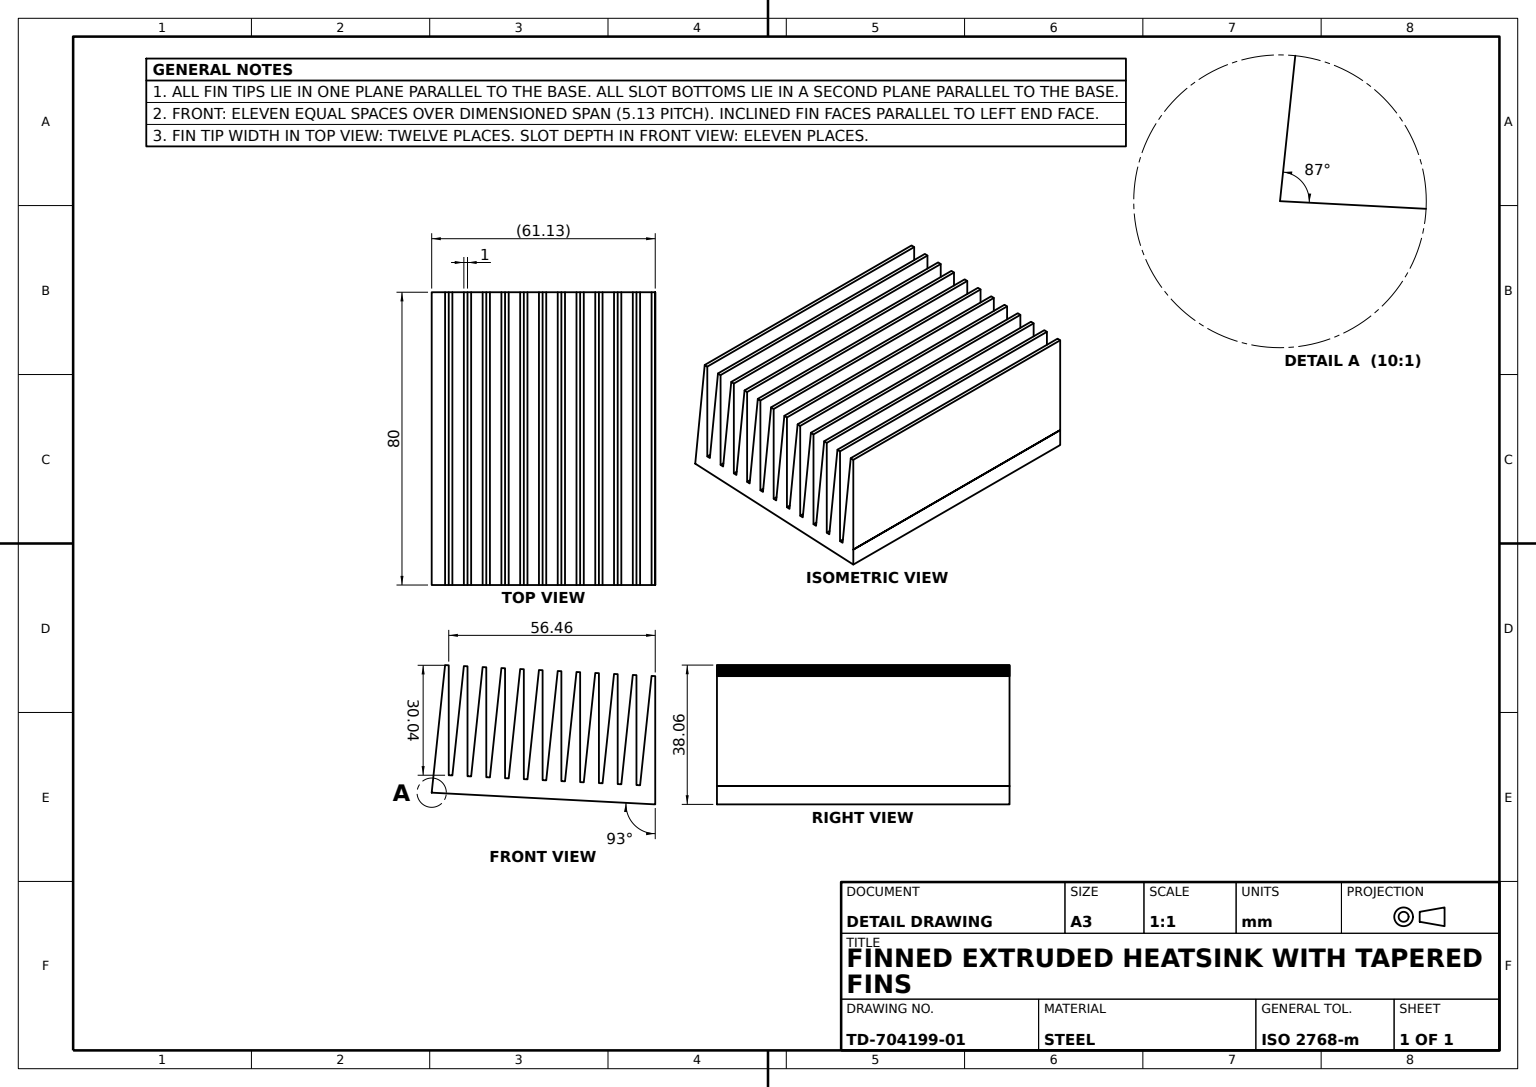
from build123d import *

# Parameters (mm, degrees)
BASE_PROFILE_SKETCH_W      = 61.21
BASE_PROFILE_SKETCH_H      = 80
HEAT_SINK_BASE_BLOCK_DEPTH = 35
FIN_SLOTS_CUT_DEPTH        = 105
SIDE_TRIM_CUT_DEPTH        = 180.145


with BuildPart() as part:
    # Base Profile Sketch → Heat Sink Base Block (new body)
    with BuildSketch(Plane(origin=(0, 0, 0), x_dir=(1, 0, 0), z_dir=(0, 1, 0))):
        with Locations((-0.605, 0)):
            Rectangle(BASE_PROFILE_SKETCH_W, BASE_PROFILE_SKETCH_H)
    extrude(amount=HEAT_SINK_BASE_BLOCK_DEPTH)

    # Fin Slots Sketch → Fin Slots Cut (cut)
    with BuildSketch(Plane.XY.offset(40)):
        Polygon((23.025727725, 35), (24.597961104, 5), (25.593494347, 5), (27.165727725, 35), align=None)
        Polygon((28.165727725, 35), (30, 0), (30, 35), align=None)
        Polygon((20.453494347, 5), (22.025727725, 35), (22.021260968, 35), (17.885727725, 35), (19.457961104, 5), align=None)
        Polygon((15.313494347, 5), (16.885727725, 35), (12.745727725, 35), (14.317961104, 5), align=None)
        Polygon((10.173494347, 5), (11.745727725, 35), (7.605727725, 35), (9.177961104, 5), align=None)
        Polygon((5.033494347, 5), (6.605727725, 35), (2.465727725, 35), (4.037961104, 5), align=None)
        Polygon((-0.106505653, 5), (1.465727725, 35), (-2.674272275, 35), (-1.102038896, 5), align=None)
        Polygon((-5.246505653, 5), (-3.674272275, 35), (-7.814272275, 35), (-6.242038896, 5), align=None)
        Polygon((-10.386505653, 5), (-8.814272275, 35), (-12.954272275, 35), (-11.382038896, 5), align=None)
        Polygon((-15.526505653, 5), (-13.954272275, 35), (-18.094272275, 35), (-16.522038896, 5), align=None)
        Polygon((-20.666505653, 5), (-19.094272275, 35), (-23.234272275, 35), (-21.662038896, 5), align=None)
        Polygon((-25.806505653, 5), (-24.234272275, 35), (-28.374272275, 35), (-26.802038896, 5), align=None)
        Polygon((-30.946505653, 5), (-29.374272275, 35), (-31.20854455, 35), (-31.20854455, 5), align=None)
    extrude(amount=-FIN_SLOTS_CUT_DEPTH, mode=Mode.SUBTRACT)

    # Side Trim Sketch → Side Trim Cut (cut)
    with BuildSketch(Plane.XY.offset(40)):
        Polygon((-29.374272275, 35), (-31.21, 0), (-36.791681348, 0), (-36.791681348, 36.336825614), (-29.374272275, 36.336825614), align=None)
    extrude(amount=-SIDE_TRIM_CUT_DEPTH, mode=Mode.SUBTRACT)


solid = part.part
